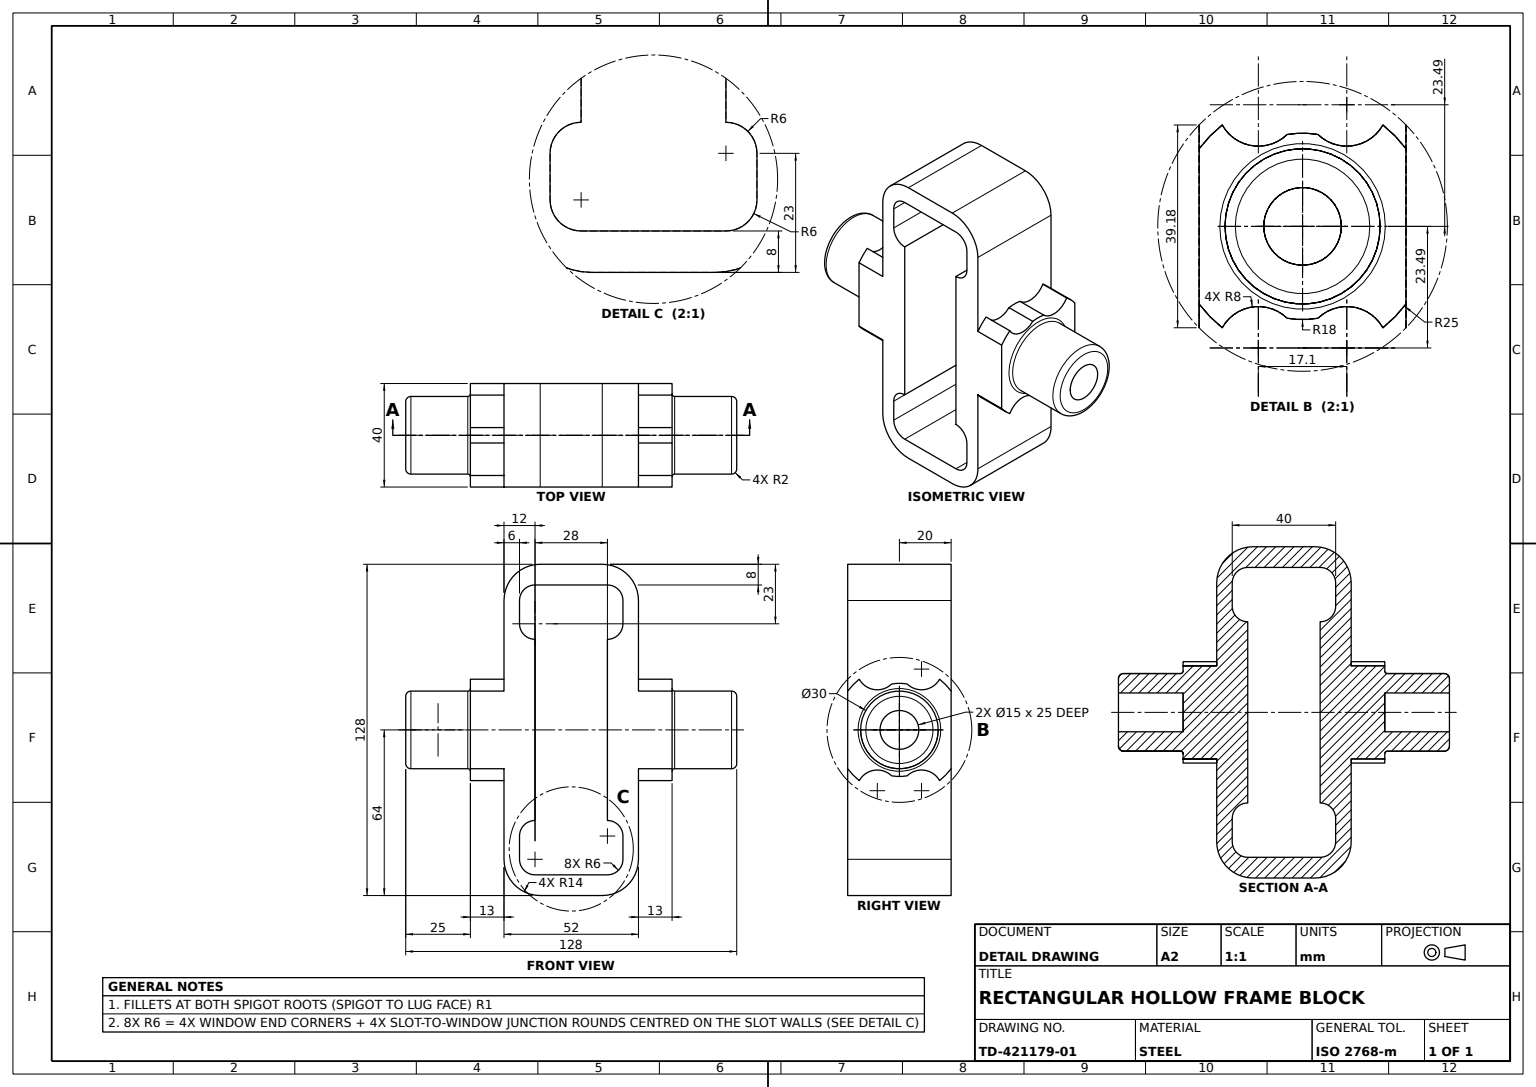
from build123d import *

# Parameters (mm, degrees)
FRAME_BODY_DEPTH         = 40
FRAME_WINDOW_CUT_DEPTH   = 40
SIDE_LUG_A_DEPTH         = 13
SPIGOT_A_SKETCH_R        = 15
SPIGOT_A_SKETCH_R_2      = 7.5
SPIGOT_A_30_DEPTH        = 25
SIDE_START               = 13
SIDE_LUG_B_DEPTH         = 13
SPIGOT_START             = 25
SPIGOT_B_SKETCH_R        = 15
SPIGOT_B_SKETCH_R_2      = 7.5
SPIGOT_B_30_DEPTH        = 25
SPIGOT_EDGE_FILLETS_R2_R = 2
LUG_BLEND_FILLETS_R1_R   = 1


with BuildPart() as part:
    # Frame Profile Sketch → Frame Body (new body)
    with BuildSketch(Plane.XY):
        with BuildLine():
            Line((-12, -64), (12, -64))
            ThreePointArc((12, -64), (21.899494937, -59.899494937), (26, -50))
            Line((26, -50), (26, 50))
            ThreePointArc((26, 50), (21.899494937, 59.899494937), (12, 64))
            Line((12, 64), (-12, 64))
            ThreePointArc((-12, 64), (-21.899494937, 59.899494937), (-26, 50))
            Line((-26, 50), (-26, -50))
            ThreePointArc((-26, -50), (-21.899494937, -59.899494937), (-12, -64))
        make_face()
    extrude(amount=FRAME_BODY_DEPTH)

    # Frame Window Sketch → Frame Window Cut (cut)
    with BuildSketch(Plane.XY.offset(40)):
        with BuildLine():
            Line((14, -35), (14, 35))
            ThreePointArc((14, 35), (18.242640687, 36.757359313), (20, 41))
            Line((20, 41), (20, 50))
            ThreePointArc((20, 50), (18.242640687, 54.242640687), (14, 56))
            Line((14, 56), (-14, 56))
            ThreePointArc((-14, 56), (-18.242640687, 54.242640687), (-20, 50))
            Line((-20, 50), (-20, 41))
            ThreePointArc((-20, 41), (-18.242640687, 36.757359313), (-14, 35))
            Line((-14, 35), (-14, -35))
            ThreePointArc((-14, -35), (-18.242640687, -36.757359313), (-20, -41))
            Line((-20, -41), (-20, -50))
            ThreePointArc((-20, -50), (-18.242640687, -54.242640687), (-14, -56))
            Line((-14, -56), (14, -56))
            ThreePointArc((14, -56), (18.242640687, -54.242640687), (20, -50))
            Line((20, -50), (20, -41))
            ThreePointArc((20, -41), (18.242640687, -36.757359313), (14, -35))
        make_face()
    extrude(amount=-FRAME_WINDOW_CUT_DEPTH, mode=Mode.SUBTRACT)

    # Side Lug A Sketch → Side Lug A (add)
    with BuildSketch(Plane(origin=(26, 0, 0), x_dir=(0, 0, -1), z_dir=(1, 0, 0))):
        with BuildLine():
            Line((-40, 15), (-40, -15))
            ThreePointArc((-40, -15), (-37.914229564, -17.437900652), (-35.533410394, -19.588597743))
            ThreePointArc((-35.533410394, -19.588597743), (-29.708548536, -15.576576016), (-22.978505654, -17.751859172))
            ThreePointArc((-22.978505654, -17.751859172), (-20, -18), (-17.021494346, -17.751859172))
            ThreePointArc((-17.021494346, -17.751859172), (-10.291451464, -15.576576016), (-4.466589606, -19.588597743))
            ThreePointArc((-4.466589606, -19.588597743), (-2.085770436, -17.437900652), (0, -15))
            Line((0, -15), (0, 15))
            ThreePointArc((0, 15), (-2.085770436, 17.437900652), (-4.466589606, 19.588597743))
            ThreePointArc((-4.466589606, 19.588597743), (-10.291451464, 15.576576016), (-17.021494346, 17.751859172))
            ThreePointArc((-17.021494346, 17.751859172), (-20, 18), (-22.978505654, 17.751859172))
            ThreePointArc((-22.978505654, 17.751859172), (-29.708548536, 15.576576016), (-35.533410394, 19.588597743))
            ThreePointArc((-35.533410394, 19.588597743), (-37.914229564, 17.437900652), (-40, 15))
        make_face()
    extrude(amount=SIDE_LUG_A_DEPTH)

    # Spigot A Sketch → Spigot A Ø30 (add)
    with BuildSketch(Plane(origin=(39, 0, 0), x_dir=(0, 0, -1), z_dir=(1, 0, 0))):
        with Locations((-20, 0)):
            Circle(SPIGOT_A_SKETCH_R)
        with Locations((-20, 0)):
            Circle(SPIGOT_A_SKETCH_R_2, mode=Mode.SUBTRACT)
    extrude(amount=SPIGOT_A_30_DEPTH)

    # Side Lug B Sketch → Side Lug B (add)
    with BuildSketch(Plane.ZY.offset(26).offset(SIDE_START)):
        with BuildLine():
            Line((0, 15), (0, -15))
            ThreePointArc((0, -15), (2.085770436, -17.437900652), (4.466589606, -19.588597743))
            ThreePointArc((4.466589606, -19.588597743), (10.291451464, -15.576576016), (17.021494346, -17.751859172))
            ThreePointArc((17.021494346, -17.751859172), (20, -18), (22.978505654, -17.751859172))
            ThreePointArc((22.978505654, -17.751859172), (29.708548536, -15.576576016), (35.533410394, -19.588597743))
            ThreePointArc((35.533410394, -19.588597743), (37.914229564, -17.437900652), (40, -15))
            Line((40, -15), (40, 15))
            ThreePointArc((40, 15), (37.914229564, 17.437900652), (35.533410394, 19.588597743))
            ThreePointArc((35.533410394, 19.588597743), (29.708548536, 15.576576016), (22.978505654, 17.751859172))
            ThreePointArc((22.978505654, 17.751859172), (20, 18), (17.021494346, 17.751859172))
            ThreePointArc((17.021494346, 17.751859172), (10.291451464, 15.576576016), (4.466589606, 19.588597743))
            ThreePointArc((4.466589606, 19.588597743), (2.085770436, 17.437900652), (0, 15))
        make_face()
    extrude(amount=-SIDE_LUG_B_DEPTH)

    # Spigot B Sketch → Spigot B Ø30 (add)
    with BuildSketch(Plane.ZY.offset(39).offset(SPIGOT_START)):
        with Locations(Location((20, 0, 0), (0, 0, 180))):
            Circle(SPIGOT_B_SKETCH_R)
        with Locations(Location((20, 0, 0), (0, 0, 180))):
            Circle(SPIGOT_B_SKETCH_R_2, mode=Mode.SUBTRACT)
    extrude(amount=-SPIGOT_B_30_DEPTH)

    # Spigot Edge Fillets R2
    spigot_edge_fillets_r2_edges = [part.edges().sort_by_distance(p)[0] for p in [
        (64, 0, 35),
        (-64, 0, 35),
    ]]
    fillet(spigot_edge_fillets_r2_edges, radius=SPIGOT_EDGE_FILLETS_R2_R)

    # Lug Blend Fillets R1
    lug_blend_fillets_r1_edges = [part.edges().sort_by_distance(p)[0] for p in [
        (39, 0, 35),
        (-39, 0, 35),
    ]]
    fillet(lug_blend_fillets_r1_edges, radius=LUG_BLEND_FILLETS_R1_R)


solid = part.part
